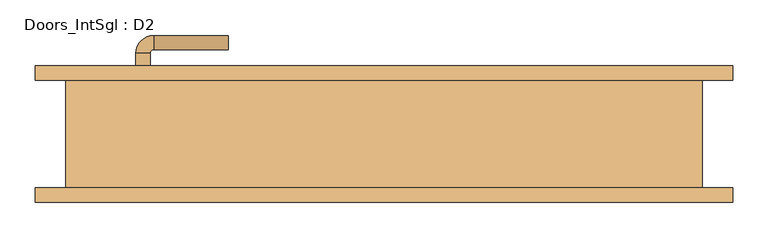
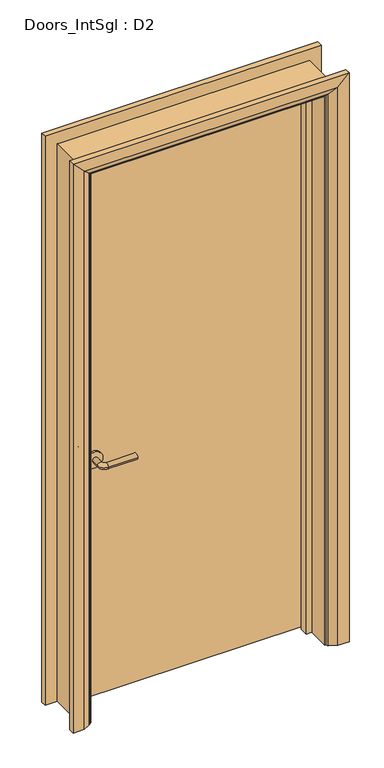
"""IFC4 building model written with IfcOpenShell, lengths in millimetres: door geometry, Doors_IntSgl : D2."""

from ifc_helpers import new_model, si_unit, point, frame, frame_2d, origin, place, context, project, spatial, polyline, circle_curve, ellipse_curve, trimmed, segment, composite_curve, outline, extrude, faceted_brep, source, transform, mapped, element, save
from ifc_brep_helpers import plane_surface, cylinder_surface, revolved_surface, advanced_brep


def doors_intsgl_d2_6b78dd6f(model_context):
    return source(origin(), model_context, "Body", "SolidModel", [
        advanced_brep(
        [(-350.2, 30.2, 900.0), (-330.2, 30.2, 900.0), (-330.2, 0.2, 900.0), (-350.2, 0.2, 900.0), (-325.2, -4.8, 900.0), (-325.2, -24.8, 900.0), (-220.2, -24.8, 900.0), (-220.2, -4.8, 900.0)],
        [
            (0, 1, circle_curve(frame((-340.2, 30.2, 900.0), z_axis=(0.0, 1.0, 0.0), x_axis=(1.0, 0.0, 0.0)), 10.0)),
            (1, 0, circle_curve(frame((-340.2, 30.2, 900.0), z_axis=(0.0, 1.0, 0.0), x_axis=(1.0, 0.0, 0.0)), 10.0)),
            (1, 2),
            (2, 3, circle_curve(frame((-340.2, 0.2, 900.0), z_axis=(0.0, 1.0, 0.0), x_axis=(1.0, 0.0, 0.0)), 10.0)),
            (3, 0),
            (3, 2, circle_curve(frame((-340.2, 0.2, 900.0), z_axis=(0.0, 1.0, 0.0), x_axis=(1.0, 0.0, 0.0)), 10.0)),
            (4, 5, circle_curve(frame((-325.2, -14.8, 900.0), z_axis=(-1.0, 0.0, 0.0), x_axis=(0.0, 1.0, 0.0)), 10.0)),
            (5, 3, circle_curve(frame((-325.2, 0.2, 900.0), z_axis=(0.0, 0.0, -1.0), x_axis=(-1.0, 0.0, 0.0)), 25.0)),
            (2, 4, circle_curve(frame((-325.2, 0.2, 900.0), z_axis=(0.0, 0.0, 1.0), x_axis=(-1.0, 0.0, 0.0)), 5.0)),
            (5, 4, circle_curve(frame((-325.2, -14.8, 900.0), z_axis=(-1.0, 0.0, 0.0), x_axis=(0.0, 1.0, 0.0)), 10.0)),
            (6, 7, circle_curve(frame((-220.2, -14.8, 900.0), z_axis=(1.0, 0.0, 0.0), x_axis=(0.0, 1.0, 0.0)), 10.0)),
            (7, 6, circle_curve(frame((-220.2, -14.8, 900.0), z_axis=(1.0, 0.0, 0.0), x_axis=(0.0, 1.0, 0.0)), 10.0)),
            (4, 7),
            (6, 5),
        ],
        [
            plane_surface(frame((-340.2, 30.2, 900.0), z_axis=(0.0, 1.0, 0.0), x_axis=(0.0, 0.0, 1.0))),
            cylinder_surface(frame((-340.2, 30.2, 900.0), z_axis=(0.0, 1.0, 0.0), x_axis=(1.0, 0.0, 0.0)), 10.0),
            revolved_surface(trimmed(ellipse_curve(frame((-340.2, 0.2, 900.0), z_axis=(0.0, -1.0, 0.0), x_axis=(1.0, 0.0, 0.0)), 10.0, 10.0), [point((-350.2, 0.2, 900.0))], [point((-330.2, 0.2, 900.0))], True, "CARTESIAN"), (-325.2, 0.2, 900.0), (0.0, 0.0, -1.0)),
            revolved_surface(trimmed(ellipse_curve(frame((-340.2, 0.2, 900.0), z_axis=(0.0, -1.0, 0.0), x_axis=(1.0, 0.0, 0.0)), 10.0, 10.0), [point((-330.2, 0.2, 900.0))], [point((-350.2, 0.2, 900.0))], True, "CARTESIAN"), (-325.2, 0.2, 900.0), (0.0, 0.0, -1.0)),
            plane_surface(frame((-220.2, -14.8, 900.0), z_axis=(1.0, 0.0, 0.0), x_axis=(0.0, 0.0, 1.0))),
            cylinder_surface(frame((-325.2, -14.8, 900.0), z_axis=(-1.0, 0.0, 0.0), x_axis=(0.0, 1.0, 0.0)), 10.0),
        ],
        [
            (0, [[1, 2]]),
            (1, [[3, 4, 5, -2]]),
            (1, [[-5, 6, -3, -1]]),
            (2, [[7, 8, -4, 9]]),
            (3, [[10, -9, -6, -8]]),
            (4, [[11, 12]]),
            (5, [[13, -11, 14, -7]]),
            (5, [[-14, -12, -13, -10]]),
        ],
    ),
        extrude(outline(composite_curve([segment(trimmed(circle_curve(frame_2d((900.0, -342.7)), 30.0), [point((900.0, -372.7))], [point((900.0, -312.7))], False, "CARTESIAN"), True, "CONTINUOUS"), segment(trimmed(circle_curve(frame_2d((900.0, -342.7)), 30.0), [point((900.0, -312.7))], [point((900.0, -372.7))], False, "CARTESIAN"), True, "CONTINUOUS")], self_intersect=False)), frame((0.0, 30.2, 0.0), z_axis=(0.0, 1.0, 0.0), x_axis=(0.0, 0.0, 1.0)), (0.0, 0.0, 1.0), 8.0),
        advanced_brep(
        [(-350.2, 84.2, 900.0), (-330.2, 84.2, 900.0), (-350.2, 114.2, 900.0), (-330.2, 114.2, 900.0), (-325.2, 119.2, 900.0), (-325.2, 139.2, 900.0), (-220.2, 139.2, 900.0), (-220.2, 119.2, 900.0)],
        [
            (0, 1, circle_curve(frame((-340.2, 84.2, 900.0), z_axis=(0.0, -1.0, 0.0), x_axis=(1.0, 0.0, 0.0)), 10.0)),
            (1, 0, circle_curve(frame((-340.2, 84.2, 900.0), z_axis=(0.0, -1.0, 0.0), x_axis=(1.0, 0.0, 0.0)), 10.0)),
            (0, 2),
            (2, 3, circle_curve(frame((-340.2, 114.2, 900.0), z_axis=(0.0, -1.0, 0.0), x_axis=(1.0, 0.0, 0.0)), 10.0)),
            (3, 1),
            (3, 2, circle_curve(frame((-340.2, 114.2, 900.0), z_axis=(0.0, -1.0, 0.0), x_axis=(1.0, 0.0, 0.0)), 10.0)),
            (4, 3, circle_curve(frame((-325.2, 114.2, 900.0), z_axis=(0.0, 0.0, 1.0), x_axis=(-1.0, 0.0, 0.0)), 5.0)),
            (2, 5, circle_curve(frame((-325.2, 114.2, 900.0), z_axis=(0.0, 0.0, -1.0), x_axis=(-1.0, 0.0, 0.0)), 25.0)),
            (5, 4, circle_curve(frame((-325.2, 129.2, 900.0), z_axis=(-1.0, 0.0, 0.0), x_axis=(0.0, -1.0, 0.0)), 10.0)),
            (4, 5, circle_curve(frame((-325.2, 129.2, 900.0), z_axis=(-1.0, 0.0, 0.0), x_axis=(0.0, -1.0, 0.0)), 10.0)),
            (6, 7, circle_curve(frame((-220.2, 129.2, 900.0), z_axis=(1.0, 0.0, 0.0), x_axis=(0.0, -1.0, 0.0)), 10.0)),
            (7, 6, circle_curve(frame((-220.2, 129.2, 900.0), z_axis=(1.0, 0.0, 0.0), x_axis=(0.0, -1.0, 0.0)), 10.0)),
            (5, 6),
            (7, 4),
        ],
        [
            plane_surface(frame((-340.2, 84.2, 900.0), z_axis=(0.0, -1.0, 0.0), x_axis=(0.0, 0.0, 1.0))),
            cylinder_surface(frame((-340.2, 84.2, 900.0), z_axis=(0.0, -1.0, 0.0), x_axis=(1.0, 0.0, 0.0)), 10.0),
            revolved_surface(trimmed(ellipse_curve(frame((-340.2, 114.2, 900.0), z_axis=(0.0, -1.0, 0.0), x_axis=(1.0, 0.0, 0.0)), 10.0, 10.0), [point((-350.2, 114.2, 900.0))], [point((-330.2, 114.2, 900.0))], True, "CARTESIAN"), (-325.2, 114.2, 900.0), (0.0, 0.0, -1.0)),
            revolved_surface(trimmed(ellipse_curve(frame((-340.2, 114.2, 900.0), z_axis=(0.0, -1.0, 0.0), x_axis=(1.0, 0.0, 0.0)), 10.0, 10.0), [point((-330.2, 114.2, 900.0))], [point((-350.2, 114.2, 900.0))], True, "CARTESIAN"), (-325.2, 114.2, 900.0), (0.0, 0.0, -1.0)),
            plane_surface(frame((-220.2, 129.2, 900.0), z_axis=(1.0, 0.0, 0.0), x_axis=(0.0, 0.0, 1.0))),
            cylinder_surface(frame((-325.2, 129.2, 900.0), z_axis=(-1.0, 0.0, 0.0), x_axis=(0.0, -1.0, 0.0)), 10.0),
        ],
        [
            (0, [[1, 2]]),
            (1, [[-1, 3, 4, 5]]),
            (1, [[-2, -5, 6, -3]]),
            (2, [[7, -4, 8, 9]]),
            (3, [[-8, -6, -7, 10]]),
            (4, [[11, 12]]),
            (5, [[-9, 13, -12, 14]]),
            (5, [[-10, -14, -11, -13]]),
        ],
    ),
        extrude(outline(composite_curve([segment(trimmed(circle_curve(frame_2d((900.0, -342.7)), 30.0), [point((900.0, -372.7))], [point((900.0, -312.7))], False, "CARTESIAN"), True, "CONTINUOUS"), segment(trimmed(circle_curve(frame_2d((900.0, -342.7)), 30.0), [point((900.0, -312.7))], [point((900.0, -372.7))], False, "CARTESIAN"), True, "CONTINUOUS")], self_intersect=False)), frame((0.0, 76.2, 0.0), z_axis=(0.0, 1.0, 0.0), x_axis=(0.0, 0.0, 1.0)), (0.0, 0.0, 1.0), 8.0),
        extrude(outline(polyline([(415.2, 38.2), (-415.2, 38.2), (-415.2, 76.2), (415.2, 76.2), (415.2, 38.2)])), frame((0.0, 0.0, 8.0), z_axis=(0.0, 0.0, 1.0), x_axis=(1.0, 0.0, 0.0)), (0.0, 0.0, 1.0), 2060.0),
        advanced_brep(
        [(492.2, 96.2, 0.0), (492.2, 76.2, 0.0), (422.2, 76.2, 0.0), (426.2, 82.2, 0.0), (452.2, 96.2, 0.0), (492.2, 96.2, 2145.0), (492.2, 76.2, 2145.0), (-492.2, 76.2, 2145.0), (-492.2, 76.2, 0.0), (-422.2, 76.2, 0.0), (-422.2, 76.2, 2075.0), (422.2, 76.2, 2075.0), (426.2, 82.2, 2079.0), (452.2, 96.2, 2105.0), (-452.2, 96.2, 2105.0), (-452.2, 96.2, 0.0), (-492.2, 96.2, 0.0), (-492.2, 96.2, 2145.0), (-426.2, 82.2, 0.0), (-426.2, 82.2, 2079.0)],
        [
            (0, 1),
            (1, 2),
            (2, 3, circle_curve(frame((430.2, 75.2, 0.0), z_axis=(0.0, 0.0, -1.0), x_axis=(1.0, 0.0, 0.0)), 8.0622577)),
            (3, 4),
            (4, 0),
            (0, 5),
            (5, 6),
            (6, 1),
            (6, 7),
            (7, 8),
            (8, 9),
            (9, 10),
            (10, 11),
            (11, 2),
            (11, 12, ellipse_curve(frame((430.2, 75.2, 2083.0), z_axis=(0.7071067811865475, 0.0, -0.7071067811865475), x_axis=(-0.7071067811865474, 0.0, -0.7071067811865476)), 11.4017543, 8.0622577)),
            (12, 3),
            (12, 13),
            (13, 4),
            (13, 14),
            (14, 15),
            (15, 16),
            (16, 17),
            (17, 5),
            (7, 17),
            (16, 8),
            (15, 18),
            (18, 9, circle_curve(frame((-430.2, 75.2, 0.0), z_axis=(0.0, 0.0, -1.0), x_axis=(-1.0, 0.0, 0.0)), 8.0622577)),
            (19, 10, ellipse_curve(frame((-430.2, 75.2, 2083.0), z_axis=(-0.7071067811865475, 0.0, -0.7071067811865475), x_axis=(-0.7071067811865474, 0.0, 0.7071067811865476)), 11.4017543, 8.0622577)),
            (18, 19),
            (14, 19),
            (19, 12),
        ],
        [
            plane_surface(frame((422.2, 76.2, 0.0), z_axis=(0.0, 0.0, -1.0), x_axis=(0.0, -1.0, 0.0))),
            plane_surface(frame((492.2, 96.2, 0.0), z_axis=(1.0, 0.0, 0.0), x_axis=(0.0, 0.0, 1.0))),
            plane_surface(frame((492.2, 76.2, 0.0), z_axis=(0.0, -1.0, 0.0), x_axis=(0.0, 0.0, 1.0))),
            cylinder_surface(frame((430.2, 75.2, 0.0), z_axis=(0.0, 0.0, -1.0), x_axis=(1.0, 0.0, 0.0)), 8.0622577),
            plane_surface(frame((426.2, 82.2, 0.0), z_axis=(-0.4740998230350126, 0.880471099922178, 0.0), x_axis=(0.0, 0.0, 1.0))),
            plane_surface(frame((452.2, 96.2, 0.0), z_axis=(0.0, 1.0, 0.0), x_axis=(0.0, 0.0, 1.0))),
            plane_surface(frame((-492.2, 96.2, 2145.0), z_axis=(-1.0, 0.0, 0.0), x_axis=(0.0, 0.0, -1.0))),
            plane_surface(frame((-422.2, 76.2, 0.0), z_axis=(0.0, 0.0, -1.0), x_axis=(0.0, -1.0, 0.0))),
            cylinder_surface(frame((-430.2, 75.2, 2075.0), z_axis=(0.0, 0.0, 1.0), x_axis=(-1.0, 0.0, 0.0)), 8.0622577),
            plane_surface(frame((-426.2, 82.2, 2079.0), z_axis=(0.47409982303501824, 0.8804710999221749, 0.0), x_axis=(0.0, 0.0, -1.0))),
            plane_surface(frame((492.2, 96.2, 2145.0), z_axis=(0.0, 0.0, 1.0), x_axis=(-1.0, 0.0, 0.0))),
            cylinder_surface(frame((422.2, 75.2, 2083.0), z_axis=(1.0, 0.0, 0.0), x_axis=(0.0, 0.0, 1.0)), 8.0622577),
            plane_surface(frame((426.2, 82.2, 2079.0), z_axis=(0.0, 0.8804710999221764, -0.4740998230350154), x_axis=(-1.0, 0.0, 0.0))),
        ],
        [
            (0, [[1, 2, 3, 4, 5]]),
            (1, [[-1, 6, 7, 8]]),
            (2, [[-2, -8, 9, 10, 11, 12, 13, 14]]),
            (3, [[-3, -14, 15, 16]]),
            (4, [[-4, -16, 17, 18]]),
            (5, [[-5, -18, 19, 20, 21, 22, 23, -6]]),
            (6, [[24, -22, 25, -10]]),
            (7, [[-21, 26, 27, -11, -25]]),
            (8, [[28, -12, -27, 29]]),
            (9, [[30, -29, -26, -20]]),
            (10, [[-7, -23, -24, -9]]),
            (11, [[-15, -13, -28, 31]]),
            (12, [[-17, -31, -30, -19]]),
        ],
    ),
        extrude(outline(polyline([(0.0, -417.2), (0.0, -398.2), (2051.0, -398.2), (2051.0, 398.2), (0.0, 398.2), (0.0, 417.2), (2070.0, 417.2), (2070.0, -417.2), (0.0, -417.2)])), frame((0.0, 4.2, 0.0), z_axis=(0.0, 1.0, 0.0), x_axis=(0.0, 0.0, 1.0)), (0.0, 0.0, 1.0), 32.0),
        advanced_brep(
        [(-492.2, -96.2, 0.0), (-492.2, -76.2, 0.0), (-422.2, -76.2, 0.0), (-426.2, -82.2, 0.0), (-452.2, -96.2, 0.0), (-492.2, -96.2, 2145.0), (-492.2, -76.2, 2145.0), (-422.2, -76.2, 2075.0), (-426.2, -82.2, 2079.0), (-452.2, -96.2, 2105.0), (492.2, -96.2, 0.0), (452.2, -96.2, 0.0), (426.2, -82.2, 0.0), (422.2, -76.2, 0.0), (492.2, -76.2, 0.0), (492.2, -96.2, 2145.0), (452.2, -96.2, 2105.0), (426.2, -82.2, 2079.0), (422.2, -76.2, 2075.0), (492.2, -76.2, 2145.0)],
        [
            (0, 1),
            (1, 2),
            (2, 3, circle_curve(frame((-430.2, -75.2, 0.0), z_axis=(0.0, 0.0, -1.0), x_axis=(-1.0, 0.0, 0.0)), 8.0622577)),
            (3, 4),
            (4, 0),
            (0, 5),
            (5, 6),
            (6, 1),
            (6, 7),
            (7, 2),
            (7, 8, ellipse_curve(frame((-430.2, -75.2, 2083.0), z_axis=(-0.7071067811865475, 0.0, -0.7071067811865475), x_axis=(0.7071067811865474, 0.0, -0.7071067811865476)), 11.4017543, 8.0622577)),
            (8, 3),
            (8, 9),
            (9, 4),
            (9, 5),
            (10, 11),
            (11, 12),
            (12, 13, circle_curve(frame((430.2, -75.2, 0.0), z_axis=(0.0, 0.0, -1.0), x_axis=(1.0, 0.0, 0.0)), 8.0622577)),
            (13, 14),
            (14, 10),
            (15, 16),
            (16, 11),
            (10, 15),
            (16, 17),
            (17, 12),
            (17, 18, ellipse_curve(frame((430.2, -75.2, 2083.0), z_axis=(0.7071067811865475, 0.0, -0.7071067811865475), x_axis=(0.7071067811865474, 0.0, 0.7071067811865476)), 11.4017543, 8.0622577)),
            (18, 13),
            (18, 19),
            (19, 14),
            (19, 15),
            (5, 15),
            (19, 6),
            (18, 7),
            (17, 8),
            (16, 9),
        ],
        [
            plane_surface(frame((-422.2, -149.0010989, 0.0), z_axis=(0.0, 0.0, -1.0), x_axis=(1.0, 0.0, 0.0))),
            plane_surface(frame((-492.2, -96.2, 0.0), z_axis=(-1.0, 0.0, 0.0), x_axis=(0.0, 0.0, 1.0))),
            plane_surface(frame((-492.2, -76.2, 0.0), z_axis=(0.0, 1.0, 0.0), x_axis=(0.0, 0.0, 1.0))),
            cylinder_surface(frame((-430.2, -75.2, 0.0), z_axis=(0.0, 0.0, -1.0), x_axis=(-1.0, 0.0, 0.0)), 8.0622577),
            plane_surface(frame((-426.2, -82.2, 0.0), z_axis=(0.4740998230350183, -0.8804710999221749, 0.0), x_axis=(0.0, 0.0, 1.0))),
            plane_surface(frame((-452.2, -96.2, 0.0), z_axis=(0.0, -1.0, 0.0), x_axis=(0.0, 0.0, 1.0))),
            plane_surface(frame((422.2, -149.0010989, 0.0), z_axis=(0.0, 0.0, -1.0), x_axis=(-1.0, 0.0, 0.0))),
            plane_surface(frame((452.2, -96.2, 2105.0), z_axis=(0.0, -1.0, 0.0), x_axis=(0.0, 0.0, -1.0))),
            plane_surface(frame((426.2, -82.2, 2079.0), z_axis=(-0.4740998230350183, -0.8804710999221749, 0.0), x_axis=(0.0, 0.0, -1.0))),
            cylinder_surface(frame((430.2, -75.2, 2075.0), z_axis=(0.0, 0.0, 1.0), x_axis=(1.0, 0.0, 0.0)), 8.0622577),
            plane_surface(frame((492.2, -76.2, 2145.0), z_axis=(0.0, 1.0, 0.0), x_axis=(0.0, 0.0, -1.0))),
            plane_surface(frame((492.2, -96.2, 2145.0), z_axis=(1.0, 0.0, 0.0), x_axis=(0.0, 0.0, -1.0))),
            plane_surface(frame((-492.2, -96.2, 2145.0), z_axis=(0.0, 0.0, 1.0), x_axis=(1.0, 0.0, 0.0))),
            plane_surface(frame((-492.2, -76.2, 2145.0), z_axis=(0.0, 1.0, 0.0), x_axis=(1.0, 0.0, 0.0))),
            cylinder_surface(frame((-422.2, -75.2, 2083.0), z_axis=(-1.0, 0.0, 0.0), x_axis=(0.0, 0.0, 1.0)), 8.0622577),
            plane_surface(frame((-426.2, -82.2, 2079.0), z_axis=(0.0, -0.8804710999221749, -0.4740998230350183), x_axis=(1.0, 0.0, 0.0))),
            plane_surface(frame((-452.2, -96.2, 2105.0), z_axis=(0.0, -1.0, 0.0), x_axis=(1.0, 0.0, 0.0))),
        ],
        [
            (0, [[1, 2, 3, 4, 5]]),
            (1, [[-1, 6, 7, 8]]),
            (2, [[-2, -8, 9, 10]]),
            (3, [[-3, -10, 11, 12]]),
            (4, [[-4, -12, 13, 14]]),
            (5, [[-5, -14, 15, -6]]),
            (6, [[16, 17, 18, 19, 20]]),
            (7, [[21, 22, -16, 23]]),
            (8, [[24, 25, -17, -22]]),
            (9, [[26, 27, -18, -25]]),
            (10, [[28, 29, -19, -27]]),
            (11, [[30, -23, -20, -29]]),
            (12, [[-7, 31, -30, 32]]),
            (13, [[-9, -32, -28, 33]]),
            (14, [[-11, -33, -26, 34]]),
            (15, [[-13, -34, -24, 35]]),
            (16, [[-15, -35, -21, -31]]),
        ],
    ),
        faceted_brep([(-417.2, 76.2, 0.0), (-417.2, -76.2, 0.0), (-449.2, -76.2, 0.0), (-449.2, 76.2, 0.0), (-417.2, 76.2, 2070.0), (-417.2, -76.2, 2070.0), (-449.2, -76.2, 2102.0), (-449.2, 76.2, 2102.0), (417.2, 76.2, 0.0), (449.2, 76.2, 0.0), (449.2, -76.2, 0.0), (417.2, -76.2, 0.0), (417.2, 76.2, 2070.0), (449.2, 76.2, 2102.0), (449.2, -76.2, 2102.0), (417.2, -76.2, 2070.0)], [[[0, 1, 2, 3]], [[1, 0, 4, 5]], [[2, 1, 5, 6]], [[3, 2, 6, 7]], [[0, 3, 7, 4]], [[8, 9, 10, 11]], [[12, 13, 9, 8]], [[13, 14, 10, 9]], [[14, 15, 11, 10]], [[15, 12, 8, 11]], [[5, 4, 12, 15]], [[6, 5, 15, 14]], [[7, 6, 14, 13]], [[4, 7, 13, 12]]]),
    ])


if __name__ == "__main__":
    model = new_model("IFC4")
    model_context = context("Model", 3, world=origin())
    ifc_project = project(units=[si_unit("LENGTHUNIT", "METRE", prefix="MILLI")], contexts=[model_context])
    site = spatial("IfcSite", under=ifc_project)
    building = spatial("IfcBuilding", under=site)
    placement = place(None, origin())
    doors_intsgl_d2_shape = doors_intsgl_d2_6b78dd6f(model_context)
    element("IfcDoor", 1, ObjectType="Doors_IntSgl : D2", at=placement, inside=building, context=model_context, shape_type="MappedRepresentation", body=[
        mapped(doors_intsgl_d2_shape, transform((0.0, 0.0, 0.0), x_axis=(1.0, 0.0, 0.0), y_axis=(0.0, 1.0, 0.0), z_axis=(0.0, 0.0, 1.0))),
    ])
    save(model, "model.ifc")

# Revit data of these elements
# Type "Doors_IntSgl : D2"
#   Type Mark = "47"
#   Type Comments = "Internal Single"
#   Operation = "SingleSwingRight"
#   Manufacturer = "Revit"
#   Keynote = "L20"
#   Description = "Internal Single Door"
#   Analytic Construction = "Metal"
#   UnderCut = 0.026247 ft
#   Tolerance = 0.006562 ft
#   Thickness = 0.124672 ft
#   Thermal Resistance (R) = 0.270117 (m²·K)/W
#   Structural Tolerance = 0.026247 ft
#   StopDepth = 0.104987 ft
#   Stop Thickness = 0.062336 ft
#   Rough Width = 3.0 ft
#   Rough Height = 6.922572 ft
#   Height to Top Lock Rail = 3.28084 ft
#   Heat Transfer Coefficient (U) = 3.7021 W/(m²·K)
#   Handle Z Distance = 2.952756 ft
#   Handle X Distance = 0.246063 ft
#   Frame Thickness = 0.104987 ft
#   Door Panel Width = 2.724409 ft
#   Door Panel Thickness = 0.124672 ft
#   Door Panel Offset = 0.0 ft
#   Height = 6.922572 ft
#   Width = 3.0 ft
#   Door Panel Height = 6.75853 ft
#   Architrave Setback = 0.016404 ft
#   Vis - Ironmongery = yes
#   Material Ironmongery = Door - Handle
#   Material Frame = Door - Frame/Mullion (1)
#   Material Door = Door - Panel
#   Material Architrave = Door - Architrave
#   Visual Light Transmittance = 0
#   Solar Heat Gain Coefficient = 0
#   Function = (empty or 0)
#   Wall Closure = (empty or 0)
# Element 1 (IfcDoor, "Doors_IntSgl : D2")
#   Materials on its faces: "Door - Architrave", "Door - Handle", "Door - Frame/Mullion (1)", "Door - Panel"
# Materials
#   "Door - Handle": colour RGB 0 0 0, transparency 0, Keynote = "P21", Cost = 0
#   "Door - Frame/Mullion (1)": class "Wood", colour RGB 212 179 113, transparency 0, Keynote = "L20", Cost = 0
#   "Door - Panel": class "Wood", colour RGB 210 159 95, transparency 0, Keynote = "L20", Cost = 0
#   "Door - Architrave": class "Wood", colour RGB 154 90 5, transparency 0, Keynote = "P20", Cost = 0
